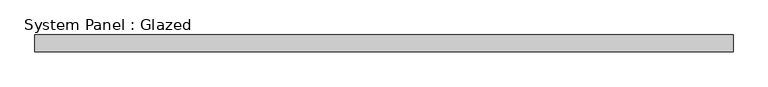
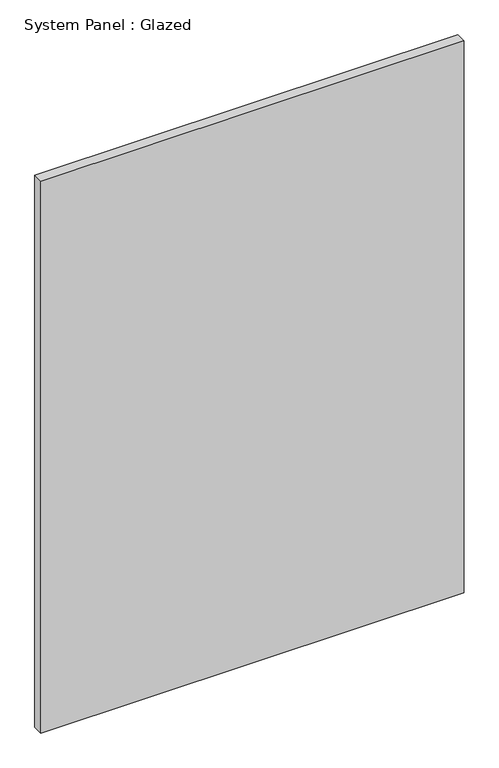
"""IFC4 building model written with IfcOpenShell, lengths in millimetres: plate geometry, System Panel : Glazed."""

from ifc_helpers import new_model, si_unit, origin, origin_with_axes, place, context, project, spatial, polyline, outline, extrude, source, transform, mapped, element, save


def system_panel_glazed_28e33a90(model_context):
    return source(origin(), model_context, "Body", "SweptSolid", [
        extrude(outline(polyline([(523.875, 19.05), (-523.875, 19.05), (-523.875, 44.45), (523.875, 44.45), (523.875, 19.05)])), origin_with_axes(), (0.0, 0.0, 1.0), 1444.0246189),
    ])


if __name__ == "__main__":
    model = new_model("IFC4")
    model_context = context("Model", 3, world=origin())
    ifc_project = project(units=[si_unit("LENGTHUNIT", "METRE", prefix="MILLI")], contexts=[model_context])
    site = spatial("IfcSite", under=ifc_project)
    building = spatial("IfcBuilding", under=site)
    placement = place(None, origin())
    system_panel_glazed_shape = system_panel_glazed_28e33a90(model_context)
    element("IfcPlate", 1, ObjectType="System Panel : Glazed", at=placement, inside=building, context=model_context, shape_type="MappedRepresentation", body=[
        mapped(system_panel_glazed_shape, transform((0.0, 0.0, 0.0), x_axis=(1.0, 0.0, 0.0), y_axis=(0.0, 1.0, 0.0), z_axis=(0.0, 0.0, 1.0))),
    ])
    save(model, "model.ifc")

# Revit data of these elements
# Type "System Panel : Glazed"
#   Construction Type Id = "GSP4R"
#   Analytic Construction = "1/8 in Pilkington single glazing"
#   Visual Light Transmittance = 0.9
#   Solar Heat Gain Coefficient = 0.86
#   Heat Transfer Coefficient (U) = 1.18115 BTU/(h·ft²·°F)
#   Define Thermal Properties by = 1
# Element 1 (IfcPlate, "System Panel : Glazed")
#   Materials on its faces: "Glass"
# Materials
#   "Glass": class "Glass", colour RGB 0 128 192, transparency 0.75, Description = "Soda Lime Glass", Cost = 0
